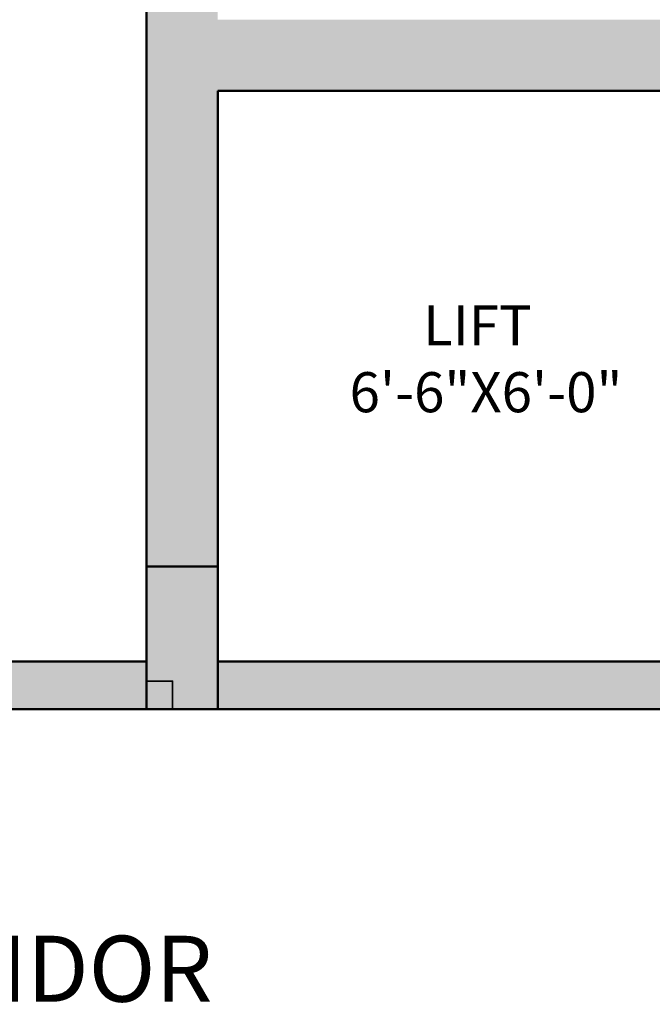
# Model space of a CAD drawing. Units: inches. Extents: x -7 to 1228, y -146 to 1091.
# Tile 62 of 88: x 531 to 611, y 531 to 655. Entities that reach past the tile are written whole.
import ezdxf

# ---------------------------------------------------------------- set-up
doc = ezdxf.new("R2010")
doc.units = ezdxf.units.IN
for name, color, linetype, lineweight in [('A-ANNO-DIMS', 2, 'Continuous', 18), ('A-ANNO-TEXT', 7, 'Continuous', 18), ('A-AREA-IDEN', 7, 'Continuous', 18), ('A-COLS', 6, 'Continuous', 35), ('A-WALL', 7, 'Continuous', 50), ('A-WALL-PATT', 251, 'Continuous', 13)]:
    doc.layers.add(name, color=color, linetype=linetype, lineweight=lineweight)
doc.styles.get("Standard").update_dxf_attribs({"font": 'arial.ttf'})
doc.dimstyles.new('ISO-25', dxfattribs={"dimtxt": 7, "dimasz": 4, "dimexe": 1.25, "dimexo": 0.625, "dimtad": 1, "dimdec": 1, "dimlunit": 3, "dimtxsty": 'Standard', "dimcen": 2.5, "dimadec": 0, "dimazin": 0, "dimtfac": 1, "dimtdec": 1, "dimtmove": 1, "dimatfit": 3, "dimfxl": 1, "dimarcsym": 0})

# ---------------------------------------------------------------- blocks, each defined once
blk = doc.blocks.new('*D49')
at = {"layer": 'A-ANNO-DIMS', "color": 0, "lineweight": -2, "transparency": 16777216}
for p, q in [((547, 676.34), (547, 670.32)), ((556, 676.34), (556, 670.32)), ((543, 671.57), (539, 671.57)), ((547, 671.57), (556, 671.57)), ((547, 671.57), (556, 671.57)), ((551.5, 671.57), (555.37, 658.66)), ((560, 671.57), (564, 671.57)), ((555.37, 658.66), (599.29, 658.66))]:
    blk.add_line(p, q, dxfattribs=at)
at = {"layer": 'A-ANNO-DIMS', "color": 0, "transparency": 16777216}
for points in [[(543, 672.23), (543, 670.9), (547, 671.57)], [(560, 672.23), (560, 670.9), (556, 671.57)]]:
    blk.add_solid(points, dxfattribs=at)
at = {"layer": 'Defpoints', "color": 0, "transparency": 16777216}
for p in [(547, 676.97), (556, 676.97), (556, 671.57)]:
    blk.add_point(p, dxfattribs=at)
at = {"layer": 'A-ANNO-DIMS', "color": 0, "transparency": 16777216, "insert": (577.33, 662.86), "char_height": 7, "attachment_point": 5}
blk.add_mtext('0\'-9" TYP.', dxfattribs=at)

msp = doc.modelspace()

# ---------------------------------------------------------------- hatches: boundary and pattern name
at = {"layer": 'A-COLS'}
h = msp.add_hatch(color=256, dxfattribs=at)
h.dxf.hatch_style = 1
h.paths.add_polyline_path([(556, 586), (547, 586), (547, 571.55), (550.29, 571.55), (550.29, 568), (556, 568)])
h = msp.add_hatch(color=256, dxfattribs=at)
h.dxf.hatch_style = 1
h.paths.add_polyline_path([(550.29, 571.55), (547, 571.55), (547, 568), (550.29, 568)])
at = {"layer": 'A-WALL-PATT'}
h = msp.add_hatch(color=256, dxfattribs=at)
h.dxf.hatch_style = 1
h.paths.add_polyline_path([(69, 568), (60, 568), (60, 493), (63.29, 493), (69, 493)])
h.paths.add_polyline_path([(69, 662.41), (60, 662.41), (60, 586), (69, 586)], flags=17)
h.paths.add_polyline_path([(69, 723), (184, 723), (184, 734), (179, 734), (179, 728), (69, 728), (69, 741.62), (60, 741.62), (60, 698.41), (69, 698.41)], flags=17)
h.paths.add_polyline_path([(69, 782), (231, 782), (231, 728), (231, 723), (231, 586), (236, 586), (236, 787), (69, 787), (69, 800.13), (60, 800.13), (60, 765.62), (69, 765.62)])
h.paths.add_polyline_path([(184, 842), (189, 842), (189, 848), (173, 848), (173, 842), (179, 842), (179, 787), (184, 787)])
h.paths.add_polyline_path([(118.22, 69), (69, 69), (69, 60), (118.22, 60)])
h.paths.add_polyline_path([(227, 69), (154.22, 69), (154.22, 60), (227, 60)])
h.paths.add_polyline_path([(236, 60), (232.71, 60), (227, 60), (227, 36), (236, 36)])
h.paths.add_polyline_path([(389, 60), (380, 60), (380, 36), (389, 36)])
h.paths.add_polyline_path([(384, 181), (380, 181), (380, 115), (380, 78), (384, 78)])
h.paths.add_polyline_path([(380, 115), (334.55, 115), (334.55, 109), (380, 109)])
h.paths.add_polyline_path([(274.55, 115), (236, 115), (236, 201), (232.71, 201), (231, 201), (231, 78), (236, 78), (236, 109), (274.55, 109)])
h.paths.add_polyline_path([(69, 123), (60, 123), (60, 78), (69, 78)])
h.paths.add_polyline_path([(69, 201), (60, 201), (60, 159), (69, 159)])
h.paths.add_polyline_path([(143, 219), (69, 219), (69, 213), (143, 213)], flags=17)
h.paths.add_polyline_path([(189, 219), (184, 219), (184, 274), (231, 274), (231, 219), (236, 219), (236, 279), (184, 279), (184, 297), (179, 297), (179, 279), (69, 279), (69, 290.91), (60, 290.91), (60, 262.18), (69, 262.18), (69, 274), (179, 274), (179, 219), (173, 219), (173, 213), (189, 213)])
h.paths.add_polyline_path([(69, 238.18), (60, 238.18), (60, 219), (69, 219)], flags=17)
h.paths.add_polyline_path([(69, 333), (60, 333), (60, 314.91), (69, 314.91), (69, 316.96)])
h.paths.add_polyline_path([(190, 338), (184, 338), (69, 338), (69, 333), (179, 333), (179, 327), (184, 327), (184, 333.02), (190, 333.05)])
h.paths.add_polyline_path([(69, 386.81), (60, 386.81), (60, 351), (69, 351)])
h.paths.add_polyline_path([(69, 475), (60, 475), (60, 422.81), (69, 422.81)])
h.paths.add_polyline_path([(236, 475), (231, 475), (231, 351.24), (236, 351.24)])
h.paths.add_polyline_path([(384, 475), (380, 475), (380, 362), (384, 362)])
h.paths.add_polyline_path([(547, 307), (439, 307), (439, 356), (445, 356), (445, 362), (433, 362), (433, 307), (380, 307), (380, 244), (380, 241), (384, 241), (384, 301), (433, 301), (433, 277), (439, 277), (439, 301), (547, 301)])
h.paths.add_polyline_path([(547, 241), (439, 241), (439, 247), (433, 247), (433, 235), (547, 235)])
h.paths.add_polyline_path([(450, 69), (440.29, 69), (424.89, 69), (389, 69), (389, 60), (450, 60)])
h.paths.add_polyline_path([(547, 69), (486, 69), (486, 60), (547, 60)])
h.paths.add_polyline_path([(556, 148.27), (547, 148.27), (547, 78), (556, 78)])
h.paths.add_polyline_path([(556, 223), (547, 223), (547, 195), (547, 184.27), (556, 184.27)])
h.paths.add_polyline_path([(556, 311.19), (547, 311.19), (547, 273.08), (556, 273.08)])
h.paths.add_polyline_path([(556, 344), (552.71, 344), (547, 344), (547, 335.19), (556, 335.19)])
h.paths.add_polyline_path([(556, 249.08), (547, 249.08), (547, 241), (556, 241)])
h.paths.add_polyline_path([(547, 362), (475, 362), (475, 356), (547, 356)], flags=0)
h.paths.add_polyline_path([(556, 399.62), (547, 399.62), (547, 362), (556, 362)])
h.paths.add_polyline_path([(556, 475), (547, 475), (547, 435.62), (556, 435.62)])
h.paths.add_polyline_path([(547, 493), (389, 493), (389, 487), (547, 487)])
h.paths.add_polyline_path([(380, 493), (278, 493), (278, 487), (380, 487)])
h.paths.add_polyline_path([(227, 493), (69, 493), (69, 487), (227, 487)])
h.paths.add_polyline_path([(643, 122.44), (634, 122.44), (634, 78), (643, 78)])
h.paths.add_polyline_path([(702.5, 69), (692.79, 69), (677.39, 69), (643, 69), (643, 60), (702.5, 60)])
h.paths.add_polyline_path([(798, 69), (738.5, 69), (738.5, 60), (798, 60)])
h.paths.add_polyline_path([(807, 60), (803.71, 60), (798, 60), (798, 36), (807, 36)])
h.paths.add_polyline_path([(807, 109), (846.75, 109), (846.75, 115), (807, 115), (807, 159), (802, 159), (802, 78), (807, 78)])
h.paths.add_polyline_path([(807, 201), (802, 201), (802, 195), (807, 195)])
h.paths.add_polyline_path([(643, 201), (634, 201), (634, 158.44), (643, 158.44)])
h.paths.add_polyline_path([(756, 225), (751, 225), (751, 219), (643, 219), (643, 213), (756, 213)])
h.paths.add_polyline_path([(643, 240.85), (634, 240.85), (634, 219), (643, 219)])
h.paths.add_polyline_path([(643, 274), (643, 288.63), (634, 288.63), (634, 264.85), (643, 264.85)])
h.paths.add_polyline_path([(802, 279), (756, 279), (756, 297), (751, 297), (751, 279), (643, 279), (643, 274), (751, 274), (751, 255), (756, 255), (756, 274), (802, 274)])
h.paths.add_polyline_path([(807, 333), (803.71, 333), (802, 333), (802, 279), (802, 274), (802, 219), (807, 219)])
h.paths.add_polyline_path([(956, 182), (951, 182), (951, 115), (906.75, 115), (906.75, 109), (951, 109), (951, 78), (956, 78)])
h.paths.add_polyline_path([(960, 60), (951, 60), (951, 36), (960, 36)])
h.paths.add_polyline_path([(1021, 69), (1005.78, 69), (960, 69), (960, 60), (1021, 60)])
h.paths.add_polyline_path([(956, 224), (951, 224), (951, 218), (956, 218)])
h.paths.add_polyline_path([(956, 302), (1004, 302), (1004, 278), (1010, 278), (1010, 302), (1118, 302), (1118, 290.81), (1127, 290.81), (1127, 326.97), (1118, 326.97), (1118, 320.97), (1118, 307), (1010, 307), (1010, 356), (1016, 356), (1016, 362), (1004, 362), (1004, 307), (951, 307), (951, 244), (951, 242), (954.29, 242), (956, 242)])
h.paths.add_polyline_path([(643, 333), (634, 333), (634, 312.63), (643, 312.63), (643, 316.96)])
h.paths.add_polyline_path([(756, 338), (643, 338), (643, 333), (751, 333), (751, 327), (756, 327)])
h.paths.add_polyline_path([(643, 388), (634, 388), (634, 351), (643, 351)])
h.paths.add_polyline_path([(807, 357), (802, 357), (802, 351), (807, 351)])
h.paths.add_polyline_path([(807, 475), (802, 475), (802, 393), (807, 393)])
h.paths.add_polyline_path([(643, 475), (634, 475), (634, 424), (643, 424)])
h.paths.add_polyline_path([(798, 493), (643, 493), (643, 487), (798, 487)])
h.paths.add_polyline_path([(634, 493), (556, 493), (556, 487), (634, 487)])
h.paths.add_polyline_path([(813, 493), (807, 493), (807, 487), (813, 487)])
h.paths.add_polyline_path([(951, 493), (849, 493), (849, 487), (951, 487)])
h.paths.add_polyline_path([(956, 484), (951, 484), (951, 374), (956, 374)])
h.paths.add_polyline_path([(1109, 493), (969, 493), (969, 487), (1109, 487)])
h.paths.add_polyline_path([(1127, 484), (1118, 484), (1118, 450.64), (1127, 450.64)])
h.paths.add_polyline_path([(1127, 414.64), (1118, 414.64), (1118, 365), (1127, 365)])
h.paths.add_polyline_path([(1109, 362), (1046, 362), (1046, 356), (1109, 356)], flags=17)
h.paths.add_polyline_path([(1127, 356), (1123.45, 356), (1118, 356), (1118, 350.97), (1127, 350.97)], flags=0)
h.paths.add_polyline_path([(1127, 266.81), (1118, 266.81), (1118, 262.36), (1118, 242), (1127, 242)], flags=17)
h.paths.add_polyline_path([(1118, 242), (1010, 242), (1010, 248), (1004, 248), (1004, 237), (1118, 237)])
h.paths.add_polyline_path([(1127, 224), (1118, 224), (1118, 170), (1127, 170)])
h.paths.add_polyline_path([(1127, 134), (1118, 134), (1118, 78), (1127, 78)])
h.paths.add_polyline_path([(1118, 69), (1057, 69), (1057, 60), (1118, 60)])
h.paths.add_polyline_path([(227, 571.55), (227, 574), (69, 574), (69, 568), (227, 568)])
h.paths.add_polyline_path([(380, 571.55), (380, 574), (278, 574), (278, 568), (380, 568)])
h.paths.add_polyline_path([(242, 574), (236, 574), (236, 568), (242, 568)])
h.paths.add_polyline_path([(547, 571.55), (547, 574), (389, 574), (389, 568), (547, 568)])
h.paths.add_polyline_path([(384, 733), (380, 733), (380, 586), (384, 586)])
h.paths.add_polyline_path([(556, 646), (634, 646), (634, 655), (547, 655), (547, 586), (556, 586)])
h.paths.add_polyline_path([(634, 574), (556, 574), (556, 568), (634, 568)])
h.paths.add_polyline_path([(643, 655), (634, 655), (634, 586), (643, 586)])
h.paths.add_polyline_path([(798, 574), (643, 574), (643, 568), (798, 568)])
h.paths.add_polyline_path([(643, 663.85), (634, 663.85), (634, 655), (643, 655)])
h.paths.add_polyline_path([(556, 676.97), (547, 676.97), (547, 655), (556, 655)])
h.paths.add_polyline_path([(556, 733), (547, 733), (547, 712.97), (556, 712.97)])
h.paths.add_polyline_path([(643, 710), (634, 710), (634, 699.85), (643, 699.85)])
h.paths.add_polyline_path([(807, 668), (802, 668), (802, 586), (807, 586)])
h.paths.add_polyline_path([(951, 574), (849, 574), (849, 568), (951, 568)])
h.paths.add_polyline_path([(956, 691), (951, 691), (951, 577), (956, 577)])
h.paths.add_polyline_path([(1109, 574), (969, 574), (969, 568), (1109, 568)])
h.paths.add_polyline_path([(1127, 643.4), (1118, 643.4), (1118, 577), (1127, 577)])
h.paths.add_polyline_path([(1127, 568), (1123.45, 568), (1118, 568), (1118, 493), (1127, 493)])
h.paths.add_polyline_path([(1127, 733), (1118, 733), (1118, 679.4), (1127, 679.4)])
h.paths.add_polyline_path([(1127, 777.35), (1118, 777.35), (1118, 770.04), (1118, 751), (1127, 751)], flags=17)
h.paths.add_polyline_path([(1118, 751), (1010, 751), (1010, 757), (1004, 757), (1004, 745), (1118, 745)])
h.paths.add_polyline_path([(956, 811), (1004, 811), (1004, 787), (1010, 787), (1010, 811), (1017.87, 811), (1017.87, 811.63, -0.414214), (1018.25, 812), (1031.98, 812, -0.414214), (1032.35, 811.63), (1032.35, 811), (1118, 811), (1118, 801.35), (1127, 801.35), (1127, 834.69), (1118, 834.69), (1118, 830.24), (1118, 817), (1010, 817), (1010, 866), (1016, 866), (1016, 872), (1004, 872), (1004, 817), (956, 817), (956, 866), (951, 866), (951, 751), (954.29, 751), (956, 751)])
h.paths.add_polyline_path([(1118, 872), (1046, 872), (1046, 866), (1118, 866)], flags=17)
h.paths.add_polyline_path([(1127, 924.71), (1118, 924.71), (1118, 884), (1127, 884)])
h.paths.add_polyline_path([(1127, 866), (1123.71, 866), (1118, 866), (1118, 858.69), (1127, 858.69)], flags=17)
h.paths.add_polyline_path([(956, 983), (951, 983), (951, 952), (807, 952), (807, 983), (802, 983), (802, 902), (807, 902), (807, 946), (951, 946), (951, 884), (956, 884)])
h.paths.add_polyline_path([(807, 842), (802, 842), (802, 787), (756, 787), (756, 806), (751, 806), (751, 787), (643, 787), (643, 782), (751, 782), (751, 764), (756, 764), (756, 782), (802, 782), (802, 728), (807, 728)])
h.paths.add_polyline_path([(756, 848), (643, 848), (643, 842), (751, 842), (751, 836), (756, 836)])
h.paths.add_polyline_path([(756, 734), (751, 734), (751, 728), (643, 728), (643, 723), (756, 723)])
h.paths.add_polyline_path([(643, 749.79), (634, 749.79), (634, 728), (637.29, 728), (643, 728)])
h.paths.add_polyline_path([(643, 805.41), (634, 805.41), (634, 773.79), (643, 773.79)])
h.paths.add_polyline_path([(643, 896.66), (634, 896.66), (634, 860), (637.29, 860), (643, 860)])
h.paths.add_polyline_path([(643, 842), (634, 842), (634, 829.41), (643, 829.41)])
h.paths.add_polyline_path([(643, 983), (634, 983), (634, 932.66), (643, 932.66)])
h.paths.add_polyline_path([(1127, 983), (1118, 983), (1118, 960.71), (1127, 960.71)])
h.paths.add_polyline_path([(1118, 1001), (1077.53, 1001), (1077.53, 992), (1118, 992)])
h.paths.add_polyline_path([(1041.53, 1001), (960, 1001), (960, 992), (1041.53, 992)])
h.paths.add_polyline_path([(960, 1025), (951, 1025), (951, 1001), (954.29, 1001), (960, 1001)])
h.paths.add_polyline_path([(807, 1025), (798, 1025), (798, 1001), (807, 1001)])
h.paths.add_polyline_path([(798, 1001), (738.5, 1001), (738.5, 992), (798, 992)])
h.paths.add_polyline_path([(702.5, 1001), (643, 1001), (643, 992), (702.5, 992)])
h.paths.add_polyline_path([(547, 1001), (499.11, 1001), (499.11, 992), (547, 992)])
h.paths.add_polyline_path([(463.11, 1001), (389, 1001), (389, 992), (463.11, 992)])
h.paths.add_polyline_path([(389, 1025), (380, 1025), (380, 1022), (380, 1001), (383.29, 1001), (389, 1001)])
h.paths.add_polyline_path([(236, 1025), (227, 1025), (227, 1001), (236, 1001)])
h.paths.add_polyline_path([(236, 983), (231, 983), (231, 860), (236, 860)])
h.paths.add_polyline_path([(274.55, 952), (236, 952), (236, 946), (274.55, 946)])
h.paths.add_polyline_path([(380, 952), (334.55, 952), (334.55, 946), (380, 946)])
h.paths.add_polyline_path([(384, 983), (380, 983), (380, 884), (383.29, 884), (384, 884)])
h.paths.add_polyline_path([(227, 1001), (155.01, 1001), (155.01, 992), (162.87, 992), (227, 992)])
h.paths.add_polyline_path([(119.01, 1001), (69, 1001), (69, 992), (119.01, 992)])
h.paths.add_polyline_path([(69, 983), (60, 983), (60, 922.99), (69, 922.99)])
h.paths.add_polyline_path([(69, 886.99), (60, 886.99), (60, 860), (63.29, 860), (69, 860)])
h.paths.add_polyline_path([(143, 848), (69, 848), (69, 842), (143, 842)])

# ---------------------------------------------------------------- linework, layer by layer
at = {"layer": 'A-COLS'}
msp.add_lwpolyline([(547, 568), (550.29, 568), (550.29, 571.55), (547, 571.55)], close=True, dxfattribs=at)
at = {"layer": 'A-WALL'}
for p, q in [((547, 745), (547, 574)), ((634, 646), (556, 646)), ((556, 646), (556, 574)), ((556, 586), (547, 586)), ((547, 586), (547, 568)), ((556, 568), (556, 586)), ((547, 574), (384, 574)), ((813, 574), (556, 574)), ((547, 568), (384, 568)), ((547, 568), (556, 568)), ((813, 568), (556, 568))]:
    msp.add_line(p, q, dxfattribs=at)

# ---------------------------------------------------------------- texts
at = {"layer": 'A-ANNO-TEXT', "insert": (430.35, 539.42), "char_height": 8.3203, "attachment_point": 1}
msp.add_mtext_dynamic_manual_height_columns('7 FEET WIDE CORRIDOR', width=225.8822, gutter_width=41.6, heights=[0], dxfattribs=at)
at = {"layer": 'A-AREA-IDEN', "insert": (571.09, 618.95), "char_height": 5.0568, "attachment_point": 1}
msp.add_mtext_dynamic_manual_height_columns('       LIFT\\P 6\'-6"X6\'-0"', width=137.2821, gutter_width=25.28, heights=[0], dxfattribs=at)

# ---------------------------------------------------------------- dimensions: what is measured, and where the dimension line sits
at = {"layer": 'A-ANNO-DIMS'}
dim = msp.add_linear_dim(base=(556, 671.57), p1=(547, 676.97), p2=(556, 676.97), text='<> TYP.', dimstyle='ISO-25', override={"dimdec": 1, "dimlfac": 1, "dimrnd": 0, "dimzin": 1, "dimdsep": 46, "dimlunit": 4, "dimfrac": 2}, dxfattribs=at)
dim.commit()
dim.dimension.update_dxf_attribs({"geometry": '*D49', "text_midpoint": (556, 662.86)})

doc.saveas('drawing.dxf')
